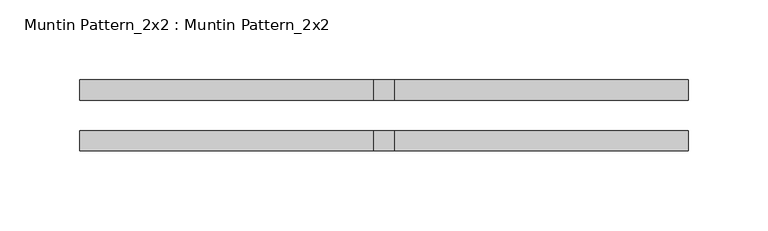
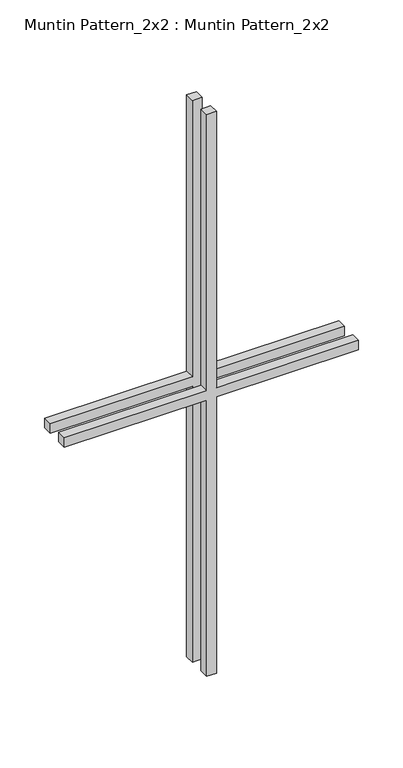
"""IFC4 building model written with IfcOpenShell, lengths in millimetres: proxy geometry, Muntin Pattern_2x2 : Muntin Pattern_2x2."""

from ifc_helpers import new_model, si_unit, frame, origin, place, context, project, spatial, polyline, outline, extrude, source, transform, mapped, element, save


def muntin_pattern_2x2_muntin_pattern_2x2_31a16349(model_context):
    return source(origin(), model_context, "Body", "SweptSolid", [
        extrude(outline(polyline([(390.525, -6.35), (390.525, -190.5), (377.825, -190.5), (377.825, -6.35), (0.0, -6.35), (0.0, 6.35), (377.825, 6.35), (377.825, 190.5), (390.525, 190.5), (390.525, 6.35), (768.35, 6.35), (768.35, -6.35), (390.525, -6.35)])), frame((0.0, 9.525, 0.0), z_axis=(0.0, 1.0, 0.0), x_axis=(0.0, 0.0, 1.0)), (0.0, 0.0, 1.0), 12.7),
        extrude(outline(polyline([(390.525, -6.35), (390.525, -190.5), (377.825, -190.5), (377.825, -6.35), (0.0, -6.35), (0.0, 6.35), (377.825, 6.35), (377.825, 190.5), (390.525, 190.5), (390.525, 6.35), (768.35, 6.35), (768.35, -6.35), (390.525, -6.35)])), frame((0.0, -22.225, 0.0), z_axis=(0.0, 1.0, 0.0), x_axis=(0.0, 0.0, 1.0)), (0.0, 0.0, 1.0), 12.7),
    ])


if __name__ == "__main__":
    model = new_model("IFC4")
    model_context = context("Model", 3, world=origin())
    ifc_project = project(units=[si_unit("LENGTHUNIT", "METRE", prefix="MILLI")], contexts=[model_context])
    site = spatial("IfcSite", under=ifc_project)
    building = spatial("IfcBuilding", under=site)
    placement = place(None, origin())
    muntin_pattern_2x2_muntin_pattern_2x2_shape = muntin_pattern_2x2_muntin_pattern_2x2_31a16349(model_context)
    element("IfcBuildingElementProxy", 1, Name="Muntin Pattern_2x2 : Muntin Pattern_2x2", ObjectType="Muntin Pattern_2x2 : Muntin Pattern_2x2", at=placement, inside=building, context=model_context, shape_type="MappedRepresentation", body=[
        mapped(muntin_pattern_2x2_muntin_pattern_2x2_shape, transform((0.0, 0.0, 0.0), x_axis=(1.0, 0.0, 0.0), y_axis=(0.0, 1.0, 0.0), z_axis=(0.0, 0.0, 1.0))),
    ])
    save(model, "model.ifc")

# Revit data of these elements
# Type "Muntin Pattern_2x2 : Muntin Pattern_2x2"
#   Width [instance default] = 4 ft
#   Thickness = 0.041667 ft
#   Height [instance default] = 4 ft
#   Distance = 0.0625 ft
#   Interior Material [instance default] = none
#   Exterior Material [instance default] = none
#   Default Elevation = 0
# Element 1 (IfcBuildingElementProxy, "Muntin Pattern_2x2 : Muntin Pattern_2x2")
#   Width = 1.25 ft
#   Height = 2.520833 ft
#   Interior Material = Wood - Stained
#   Exterior Material = Clad - White
#   Materials on its faces: "Clad - White", "Wood - Stained"
# Materials
#   "Clad - White": class "Wood", colour RGB 242 242 238, transparency 0, Cost = 0
#   "Wood - Stained": class "Wood", colour RGB 224 178 126, transparency 0, Cost = 0
